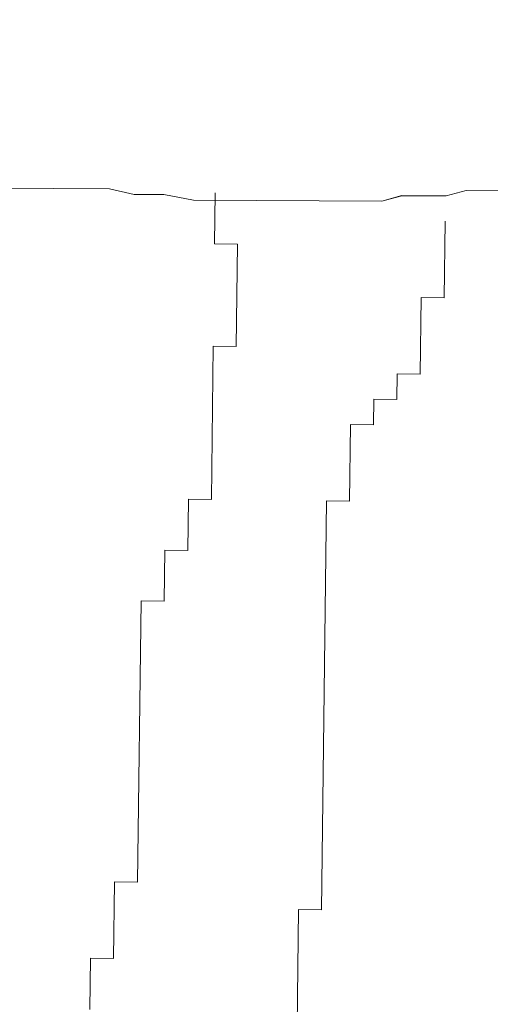
# Model space of a CAD drawing. Units: inches. Extents: x -466983 to 1020, y 324 to 318697.
# Tile 72 of 97: x 647.874 to 650.415, y 942.656 to 947.975. Entities that reach past the tile are written whole.
import ezdxf

# ---------------------------------------------------------------- set-up
doc = ezdxf.new("R2010")
doc.units = ezdxf.units.IN
doc.header["$MEASUREMENT"] = 0
doc.layers.add('A-FLOR-PATT', color=252, linetype='Continuous', lineweight=13)
doc.layers.add('A-FURN', color=8, linetype='Continuous', lineweight=18)

# ---------------------------------------------------------------- blocks, each defined once
blk = doc.blocks.new('L Shaped Sofa')
at = {"ltscale": 2}
for p, q in [((2408.5493, 742.876), (2408.5678, 744.3875)), ((2410.597, 743.3549), (2410.6031, 743.8587)), ((2410.3609, 742.602), (2410.3701, 743.3577)), ((2410.3701, 743.3577), (2410.597, 743.3549)), ((2408.2732, 738.8482), (2408.3225, 742.8788)), ((2408.3225, 742.8788), (2408.5493, 742.876)), ((2410.1002, 739.8337), (2410.1341, 742.6047)), ((2410.1341, 742.6047), (2410.3609, 742.602)), ((2409.8672, 739.3326), (2409.8734, 739.8365)), ((2409.8734, 739.8365), (2410.1002, 739.8337)), ((2409.6342, 738.8316), (2409.6404, 739.3354)), ((2409.6404, 739.3354), (2409.8672, 739.3326)), ((2408.0371, 738.0953), (2408.0464, 738.851)), ((2408.0464, 738.851), (2408.2732, 738.8482)), ((2409.3889, 737.3229), (2409.4074, 738.8344)), ((2409.4074, 738.8344), (2409.6342, 738.8316)), ((2407.8072, 737.8461), (2407.8103, 738.098)), ((2407.8103, 738.098), (2408.0371, 738.0953)), ((2407.5773, 737.597), (2407.5804, 737.8489)), ((2407.5804, 737.8489), (2407.8072, 737.8461)), ((2407.3412, 736.844), (2407.3505, 737.5998)), ((2407.3505, 737.5998), (2407.5773, 737.597)), ((2409.1498, 736.318), (2409.1621, 737.3257)), ((2409.1621, 737.3257), (2409.3889, 737.3229)), ((2407.1052, 736.0911), (2407.1144, 736.8468)), ((2407.1144, 736.8468), (2407.3412, 736.844)), ((2409.3766, 736.3153), (2409.1498, 736.318)), ((2409.3705, 735.8114), (2409.3766, 736.3153)), ((2407.5327, 735.8401), (2407.7282, 735.8934)), ((2407.7282, 735.8934), (2409.5825, 735.8847)), ((2409.5825, 735.8847), (2409.8749, 735.8291)), ((2402.3601, 735.8101), (2406.8981, 735.7888)), ((2406.8981, 735.7888), (2407.0936, 735.8421)), ((2407.0936, 735.8421), (2407.5327, 735.8401)), ((2409.8749, 735.8291), (2410.1677, 735.8277)), ((2410.1677, 735.8277), (2410.4113, 735.7723)), ((2410.4113, 735.7723), (2411.8264, 735.7657))]:
    blk.add_line(p, q, dxfattribs=at)

msp = doc.modelspace()

# ---------------------------------------------------------------- hatches: boundary and pattern name
at = {"layer": 'A-FLOR-PATT', "transparency": 33554572}
h = msp.add_hatch(dxfattribs=at)
h.set_pattern_fill('ANSI37', color=256, scale=30)
h.set_pattern_definition([(45, (-1212.4137, -290.035), (-2.6516504, 2.6516504), []), (135, (-1212.4137, -290.035), (-2.6516504, -2.6516504), [])])
h.paths.add_polyline_path([(901.8057, 1075.9377), (900.6144, 1075.9377), (900.6144, 1065.3856), (899.391, 1065.3856), (898.0911, 1065.3856), (892.8356, 1058.7098, -0.258377), (892.1875, 1058.3509), (879.9848, 1058.3509, -0.20177), (879.4382, 1058.5808), (874.0812, 1065.3856), (872.7813, 1065.3856), (871.5579, 1065.3856), (871.5579, 1075.9377), (813.8057, 1075.9377), (813.8057, 1044.7922), (832.3947, 1044.7922, -0.394795), (848.6602, 1028.5356), (848.6602, 1009.9377), (901.8057, 1009.9377), (901.8057, 1015.9377), (901.3057, 1015.9377), (871.3057, 1015.9377), (871.3057, 1017.2502), (871.3344, 1017.2502, -0.401453), (901.3057, 1045.9377), (901.8057, 1045.9377)])
edge = h.paths.add_edge_path(flags=16)
edge.add_line((847.7731, 1068.9486), (847.7731, 1073.7088))
edge.add_arc((849.2269, 1073.7088), 1.4538, 90, 180, ccw=False)
edge.add_line((849.2269, 1075.1627), (864.4921, 1075.1627))
edge.add_arc((864.4921, 1073.7088), 1.4538, 0, 90, ccw=False)
edge.add_line((865.9459, 1073.7088), (865.9459, 1069.0035))
edge.add_arc((832.6447, 1068.9761), 33.3012, -20.61234, 0.04725, ccw=False)
edge.add_ellipse((856.8595, 1058.48), major_axis=(0, 10.2131), ratio=0.6859192, start_angle=100.00884, end_angle=259.99116, ccw=False)
edge.add_arc((881.0742, 1068.9761), 33.3012, 180.04725, 200.61234, ccw=False)
h.paths.add_polyline_path([(853.1456, 1066.4815), (853.1456, 1066.4534), (853.1463, 1066.4534, 0.433107), (852.9166, 1066.6849), (852.9166, 1066.4534), (853.1456, 1066.4534), (853.1456, 1066.4815), (853.088, 1066.6122, 0.697939), (852.6995, 1066.4534), (852.7003, 1066.4534), (852.7003, 1066.4815), (852.9166, 1067.0012), (852.9166, 1066.6849, -0.396254)], flags=0)
h.paths.add_polyline_path([(861.0187, 1066.4815), (861.0187, 1066.4534), (861.0194, 1066.4534, 0.416404), (860.8024, 1066.6849), (860.8024, 1066.4534), (861.0187, 1066.4534), (861.0187, 1066.4815), (860.9672, 1066.6053, 0.713344), (860.5726, 1066.4534), (860.5734, 1066.4534), (860.5734, 1066.4815), (860.8024, 1067.0012), (860.8024, 1066.6849, -0.379973)], flags=0)
edge = h.paths.add_edge_path(flags=0)
edge.add_spline(control_points=[(861.1298, 1065.7855), (861.4661, 1065.2478), (861.6134, 1065.0161), (861.9833, 1064.3736), (862.1924, 1063.9443), (862.5614, 1063.0391), (862.7212, 1062.5633), (862.9865, 1061.5781), (863.092, 1061.0689), (863.2452, 1060.031), (863.293, 1059.5025), (863.3295, 1058.4409), (863.3181, 1057.9078), (863.2366, 1056.8518), (863.1664, 1056.3289), (862.9695, 1055.308), (862.8427, 1054.8099), (862.5365, 1053.8522), (862.3571, 1053.3927), (861.9514, 1052.5249), (861.7251, 1052.1166), (861.233, 1051.3622), (860.9672, 1051.0162), (860.4048, 1050.3949), (860.1082, 1050.1197), (859.4937, 1049.6461), (859.1758, 1049.4476), (858.5276, 1049.1299), (858.1973, 1049.0107), (857.5315, 1048.8518), (857.1959, 1048.8121), (856.5249, 1048.812), (856.1894, 1048.8515), (855.5236, 1049.0101), (855.1933, 1049.1291), (854.545, 1049.4465), (854.2271, 1049.6449), (853.6124, 1050.1183), (853.3158, 1050.3933), (852.7533, 1051.0143), (852.4874, 1051.3602), (851.9952, 1052.1144), (851.7688, 1052.5225), (851.3629, 1053.3902), (851.1834, 1053.8496), (850.877, 1054.8071), (850.7501, 1055.3051), (850.553, 1056.326), (850.4827, 1056.8488), (850.401, 1057.9048), (850.3895, 1058.4379), (850.4257, 1059.4995), (850.4734, 1060.0281), (850.6265, 1061.066), (850.7318, 1061.5753), (850.9969, 1062.5605), (851.1567, 1063.0365), (851.5254, 1063.9418), (851.7345, 1064.3712), (852.1056, 1065.0164), (852.2544, 1065.2503), (852.6082, 1065.7335)], knot_values=[3.915332, 3.915332, 3.915332, 3.915332, 4.013468, 4.013468, 4.175532, 4.175532, 4.337596, 4.337596, 4.49966, 4.49966, 4.661724, 4.661724, 4.823788, 4.823788, 4.985852, 4.985852, 5.147916, 5.147916, 5.30998, 5.30998, 5.472044, 5.472044, 5.634109, 5.634109, 5.796173, 5.796173, 5.958237, 5.958237, 6.120301, 6.120301, 6.282365, 6.282365, 6.444429, 6.444429, 6.606493, 6.606493, 6.768557, 6.768557, 6.930621, 6.930621, 7.092685, 7.092685, 7.254749, 7.254749, 7.416813, 7.416813, 7.578878, 7.578878, 7.740942, 7.740942, 7.903006, 7.903006, 8.06507, 8.06507, 8.227134, 8.227134, 8.389198, 8.389198, 8.551262, 8.551262, 8.65037, 8.65037, 8.65037, 8.65037], degree=3, periodic=0)
edge.add_line((852.6421, 1065.7855), (861.1298, 1065.7855))
edge = h.paths.add_edge_path(flags=0)
edge.add_ellipse((856.8496, 1057.7432), major_axis=(0, 7.7921), ratio=0.687861, start_angle=0, end_angle=360)
h.paths.add_polyline_path([(848.8634, 1069.3891), (848.8634, 1073.9605, -0.414214), (849.9538, 1075.0508), (863.7652, 1075.0508, -0.414214), (864.8555, 1073.9605), (864.8555, 1069.3891, -0.388936), (864.5237, 1069.027, -0.043561), (849.1953, 1069.027, -0.388936)], flags=0)
h.paths.add_polyline_path([(853.1006, 1068.1122, -1), (852.6775, 1068.1122, -1)], flags=0)
edge = h.paths.add_edge_path(flags=0)
edge.add_ellipse((856.8595, 1057.3378), major_axis=(0, 2.207), ratio=0.657164, start_angle=0, end_angle=360)
h.paths.add_polyline_path([(861.0415, 1068.1122, -1), (860.6184, 1068.1122, -1)], flags=0)
edge = h.paths.add_edge_path()
edge.add_line((573.9537, 1057.3412), (573.9537, 1075.9377))
edge.add_line((573.9537, 1075.9377), (558.7308, 1075.9377))
edge.add_line((558.7308, 1075.9377), (558.7308, 1065.3856))
edge.add_line((558.7308, 1065.3856), (557.5074, 1065.3856))
edge.add_line((557.5074, 1065.3856), (556.2075, 1065.3856))
edge.add_line((556.2075, 1065.3856), (550.952, 1058.7098))
edge.add_arc((550.3039, 1059.1155), 0.7646, 270, 327.9483, ccw=False)
edge.add_line((550.3039, 1058.3509), (538.1012, 1058.3509))
edge.add_arc((538.1012, 1059.1155), 0.7646, 224.3704, 270, ccw=False)
edge.add_line((537.5546, 1058.5808), (532.1976, 1065.3856))
edge.add_line((532.1976, 1065.3856), (530.8977, 1065.3856))
edge.add_line((530.8977, 1065.3856), (529.6743, 1065.3856))
edge.add_line((529.6743, 1065.3856), (529.6743, 1075.9377))
edge.add_line((529.6743, 1075.9377), (520.8057, 1075.9377))
edge.add_line((520.8057, 1075.9377), (520.8057, 1045.9377))
edge.add_line((520.8057, 1045.9377), (521.3057, 1045.9377))
edge.add_arc((521.3057, 1015.9377), 30, 2.50749, 90, ccw=False)
edge.add_line((551.277, 1017.2502), (551.3057, 1017.2502))
edge.add_line((551.3057, 1017.2502), (551.3057, 1015.9377))
edge.add_line((551.3057, 1015.9377), (520.8057, 1015.9377))
edge.add_line((520.8057, 1015.9377), (520.8057, 1009.9377))
edge.add_line((520.8057, 1009.9377), (559.1913, 1010.4022))
edge.add_arc((559.1913, 1011.856), 1.4538, 180, 270, ccw=False)
edge.add_line((557.7375, 1011.856), (557.7375, 1016.5613))
edge.add_arc((591.0386, 1016.5888), 33.3012, 159.38766, 180.04725, ccw=False)
edge.add_ellipse((566.8239, 1027.0848), major_axis=(0, 10.2131), ratio=0.6859192, start_angle=280.00884, end_angle=439.99116, ccw=False)
edge.add_arc((542.6091, 1016.5888), 33.3012, 0.04725, 20.61234, ccw=False)
edge.add_line((575.9103, 1016.6162), (575.9103, 1011.856))
edge.add_arc((574.4565, 1011.856), 1.4538, -90, 0, ccw=False)
edge.add_line((574.4565, 1010.4022), (608.8057, 1009.9377))
edge.add_line((608.8057, 1009.9377), (608.8057, 1041.0857))
edge.add_line((608.8057, 1041.0857), (590.2179, 1041.0857))
edge.add_arc((590.775, 1057.9074), 16.8309, 181.92775, 268.10321, ccw=False)
edge = h.paths.add_edge_path()
edge.add_ellipse((494.2443, 583.6204), major_axis=(0, 10.2131), ratio=0.6859192, start_angle=280.00884, end_angle=439.99116, ccw=False)
edge.add_arc((470.0296, 573.1243), 33.3012, 0.04725, 20.61234, ccw=False)
edge.add_line((503.3307, 573.1518), (503.3307, 568.3916))
edge.add_arc((501.8769, 568.3916), 1.4538, -90, 0, ccw=False)
edge.add_line((501.8769, 566.9377), (539.8057, 566.9377))
edge.add_line((539.8057, 566.9377), (539.8057, 572.9377))
edge.add_line((539.8057, 572.9377), (539.3057, 572.9377))
edge.add_line((539.3057, 572.9377), (509.3057, 572.9377))
edge.add_line((509.3057, 572.9377), (509.3057, 574.2502))
edge.add_line((509.3057, 574.2502), (509.3344, 574.2502))
edge.add_arc((539.3057, 572.9377), 30, 90, 177.49251, ccw=False)
edge.add_line((539.3057, 602.9377), (539.8057, 602.9377))
edge.add_line((539.8057, 602.9377), (539.8057, 626.9377))
edge.add_line((539.8057, 626.9377), (531.7718, 626.9377))
edge.add_line((531.7718, 626.9377), (531.7718, 616.3856))
edge.add_line((531.7718, 616.3856), (530.5484, 616.3856))
edge.add_line((530.5484, 616.3856), (529.2485, 616.3856))
edge.add_line((529.2485, 616.3856), (523.7105, 609.3509))
edge.add_line((523.7105, 609.3509), (510.7766, 609.3509))
edge.add_line((510.7766, 609.3509), (505.2386, 616.3856))
edge.add_line((505.2386, 616.3856), (503.9387, 616.3856))
edge.add_line((503.9387, 616.3856), (502.7153, 616.3856))
edge.add_line((502.7153, 616.3856), (502.7153, 626.9377))
edge.add_line((502.7153, 626.9377), (481.6983, 626.9377))
edge.add_line((481.6983, 626.9377), (481.6983, 610.995))
edge.add_arc((467.2703, 611.4728), 14.4359, 271.92775, 358.10321, ccw=False)
edge.add_line((467.7559, 597.0451), (451.8057, 597.0451))
edge.add_line((451.8057, 597.0451), (451.8057, 584.4035))
edge.add_line((451.8057, 584.4035), (451.8057, 566.9377))
edge.add_line((451.8057, 566.9377), (486.6117, 566.9377))
edge.add_arc((486.6117, 568.3916), 1.4538, 180, 270, ccw=False)
edge.add_line((485.1579, 568.3916), (485.1579, 573.0969))
edge.add_arc((518.4591, 573.1243), 33.3012, 159.38766, 180.04725, ccw=False)
h.paths.add_polyline_path([(836.2609, 1020.7328), (879.8898, 1020.7328), (879.8898, 1039.3902), (836.2609, 1039.3902)], flags=25)
h.paths.add_polyline_path([(549.9851, 1036.7492), (593.614, 1036.7492), (593.614, 1055.4065), (549.9851, 1055.4065)], flags=24)
h.paths.add_polyline_path([(475.123, 595.5959), (518.752, 595.5959), (518.752, 614.2532), (475.123, 614.2532)], flags=24)
h = msp.add_hatch(dxfattribs=at)
h.set_pattern_fill('ANSI37', color=256, scale=20)
h.set_pattern_definition([(45, (-1212.4137, -290.035), (-1.767767, 1.767767), []), (135, (-1212.4137, -290.035), (-1.767767, -1.767767), [])])
h.paths.add_polyline_path([(809.8057, 870.9377), (809.8057, 888.1519), (806.9985, 888.1519), (802.6624, 888.1519), (789.3832, 888.1519), (786.2846, 888.1519, -0.414214), (785.4991, 888.9374), (785.4991, 900.1959), (785.4991, 908.4696, -0.414214), (786.8082, 909.7787, -0.414214), (785.4991, 911.0878), (785.4991, 929.1015, -0.414214), (786.8082, 930.4106, -0.414214), (785.4991, 931.7197), (785.4991, 931.9039, -0.414214), (784.19, 930.5948), (766.7223, 930.5948, -0.412359), (765.4132, 931.8956, -0.413741), (764.1145, 930.5782), (744.5781, 930.422, -0.416556), (743.7864, 931.2075), (743.7864, 933.5153), (742.2154, 933.5153), (742.2154, 952.024, -0.001344), (743.7864, 952.1998), (743.7864, 953.9377), (678.5915, 953.9377), (678.5915, 951.1305), (678.5915, 946.7945), (678.5915, 933.5153), (678.5915, 930.4166, -0.414214), (677.806, 929.6312), (666.5475, 929.6312), (658.2738, 929.6312, -0.414214), (656.9647, 930.9403, -0.414214), (655.6556, 929.6312), (637.6419, 929.6312, -0.414214), (636.3328, 930.9403, -0.414214), (635.0237, 929.6312), (634.8395, 929.6312, -0.414214), (636.1486, 928.322), (636.1486, 910.8544, -0.412359), (634.8478, 909.5452, -0.413741), (636.1653, 908.2466), (636.3214, 888.7102, -0.416556), (635.5359, 887.9184), (633.2281, 887.9184), (633.2281, 886.3475), (614.7194, 886.3475, -0.001344), (614.5436, 887.9184), (612.8057, 887.9184), (612.8057, 834.9377), (612.8057, 752.9377), (612.8057, 748.9377), (612.8057, 697.9377), (654.8057, 697.9377), (654.8057, 701.9377), (715.8057, 701.9377), (715.8057, 737.4353), (774.2918, 737.4353), (774.2918, 795.9377), (809.8057, 795.9377)])
h.paths.add_polyline_path([(679.2761, 849.5757, 0.102523), (682.1475, 849.2608, -0.080461), (694.5428, 849.7725, -0.283899), (694.4822, 849.0082, 0.136605), (694.4068, 848.8103, -0.030441), (694.5428, 846.8929), (694.5428, 842.6198), (694.5428, 838.3466, -0.028219), (694.4246, 836.5684), (694.425, 836.5684, 0.196187), (694.4456, 836.2708, -0.302897), (694.5428, 835.467, -0.080461), (682.1475, 835.9787, 0.102523), (679.2761, 835.6638, -0.58611), (678.6457, 836.0169), (678.6457, 849.2227, -0.58611)], flags=16)
h.paths.add_polyline_path([(679.5173, 848.6515, 0.699597), (679.476, 848.6342, 1.20716), (679.1935, 848.7422, 0.010621)], flags=0)
h.paths.add_polyline_path([(679.4923, 836.5608, -0.013798), (679.9178, 836.6594, -0.071703), (682.8533, 837.1434, -0.165743), (682.1665, 839.1006), (682.1665, 842.6094), (682.1665, 846.0603, -0.240616), (683.4733, 848.6767, -0.068263), (693.9295, 849.0082), (693.7875, 848.7083), (693.7875, 849.0228, 0.067332), (683.4733, 848.6767, 0.240616), (682.1665, 846.0603), (682.1665, 842.6094), (682.1665, 839.1006, 0.23459), (683.461, 836.5513, 0.068093), (693.7875, 836.1955), (693.7875, 836.5104), (693.9296, 836.2102, -0.077215), (682.2421, 836.7815, 0.086627), (679.5283, 836.5701, -0.628402), (679.5029, 836.5735), (679.5029, 836.6071, 0.910458)], flags=0)
h.paths.add_polyline_path([(679.476, 848.6364), (679.2069, 848.647), (679.2069, 836.5718, 0.913566), (679.3645, 836.5861), (679.476, 836.5824)], flags=0)
h.paths.add_polyline_path([(679.2761, 829.8604, 0.102523), (682.1475, 829.5455, -0.080461), (694.5428, 830.0572, -0.283899), (694.4822, 829.2929, 0.136605), (694.4068, 829.095, -0.030441), (694.5428, 827.1776), (694.5428, 822.9045), (694.5428, 818.6314, -0.028219), (694.4246, 816.8531), (694.425, 816.8532, 0.196187), (694.4456, 816.5555, -0.302897), (694.5428, 815.7517, -0.080461), (682.1475, 816.2635, 0.102523), (679.2761, 815.9485, -0.58611), (678.6457, 816.3016), (678.6457, 829.5074, -0.58611)], flags=16)
h.paths.add_polyline_path([(679.5173, 828.9362, 0.699597), (679.476, 828.9189, 1.20716), (679.1935, 829.0269, 0.010621)], flags=0)
h.paths.add_polyline_path([(679.4923, 816.8456, -0.013798), (679.9178, 816.9441, -0.071703), (682.8533, 817.4281, -0.165743), (682.1665, 819.3853), (682.1665, 822.8941), (682.1665, 826.345, -0.240616), (683.4733, 828.9614, -0.068263), (693.9295, 829.2929), (693.7875, 828.9931), (693.7875, 829.3076, 0.067332), (683.4733, 828.9614, 0.240616), (682.1665, 826.345), (682.1665, 822.8941), (682.1665, 819.3853, 0.23459), (683.461, 816.836, 0.068093), (693.7875, 816.4802), (693.7875, 816.7952), (693.9296, 816.4949, -0.077215), (682.2421, 817.0662, 0.086627), (679.5283, 816.8549, -0.628402), (679.5029, 816.8582), (679.5029, 816.8918, 0.910458)], flags=0)
h.paths.add_polyline_path([(679.476, 828.9211), (679.2069, 828.9317), (679.2069, 816.8565, 0.913566), (679.3645, 816.8708), (679.476, 816.8671)], flags=0)
h.paths.add_polyline_path([(679.2761, 810.1451, 0.102523), (682.1475, 809.8302, -0.080461), (694.5428, 810.342, -0.3023), (694.4466, 809.5394, 0.10023), (694.4058, 809.3878, -0.03057), (694.5428, 807.4623), (694.5428, 803.1892), (694.5428, 798.9161, -0.03057), (694.4058, 796.9906, 0.10023), (694.4466, 796.839, -0.3023), (694.5428, 796.0365, -0.080461), (682.1475, 796.5482, 0.102523), (679.2761, 796.2333, -0.58611), (678.6457, 796.5863), (678.6457, 809.7921, -0.58611)], flags=16)
h.paths.add_polyline_path([(679.5173, 809.2417, 0.699597), (679.476, 809.2244, 1.20716), (679.1935, 809.3324, 0.010621)], flags=0)
h.paths.add_polyline_path([(679.4923, 797.151, -0.013798), (679.9178, 797.2496, -0.071703), (682.8533, 797.7336, -0.165743), (682.1665, 799.6908), (682.1665, 803.1996), (682.1665, 806.6505, -0.239349), (683.461, 809.2577, -0.072465), (694.4468, 809.5405, 0.197932), (694.425, 809.2405), (693.7875, 809.2985), (693.7875, 809.6135, 0.068093), (683.461, 809.2577, 0.239349), (682.1665, 806.6505), (682.1665, 803.1996), (682.1665, 799.6908, 0.235854), (683.4733, 797.1323, 0.067332), (693.7875, 796.7861), (693.7875, 797.1006), (694.425, 797.1586, 0.197932), (694.4468, 796.8586, -0.080419), (682.1557, 797.3795, 0.083867), (679.5283, 797.1603, -0.628402), (679.5029, 797.1637), (679.5029, 797.1973, 0.910458)], flags=0)
h.paths.add_polyline_path([(679.2069, 809.2372), (679.2069, 797.162, 0.913566), (679.3645, 797.1763), (679.476, 797.1726), (679.476, 809.2266)], flags=0)
h.paths.add_polyline_path([(695.3643, 853.2989), (728.2231, 853.2989), (728.2231, 771.1519), (695.3643, 771.1519)], flags=16)
h.paths.add_polyline_path([(696.0215, 852.6417), (727.5659, 852.6417), (727.5659, 771.809), (696.0215, 771.809)], flags=0)
h.paths.add_polyline_path([(679.2761, 788.7869, 0.102523), (682.1475, 788.472, -0.080461), (694.5428, 788.9837, -0.3023), (694.4466, 788.1812, 0.10023), (694.4058, 788.0296, -0.03057), (694.5428, 786.1041), (694.5428, 781.831), (694.5428, 777.5578, -0.03057), (694.4058, 775.6323, 0.10023), (694.4466, 775.4808, -0.3023), (694.5428, 774.6782, -0.080461), (682.1475, 775.19, 0.102523), (679.2761, 774.875, -0.58611), (678.6457, 775.2281), (678.6457, 788.4339, -0.58611)], flags=16)
h.paths.add_polyline_path([(679.5173, 787.8834, 0.699597), (679.476, 787.8662, 1.20716), (679.1935, 787.9742, 0.010621)], flags=0)
h.paths.add_polyline_path([(679.4923, 775.7928, -0.013798), (679.9178, 775.8914, -0.071703), (682.8533, 776.3753, -0.165743), (682.1665, 778.3325), (682.1665, 781.8414), (682.1665, 785.2922, -0.239349), (683.461, 787.8995, -0.072465), (694.4468, 788.1823, 0.197932), (694.425, 787.8823), (693.7875, 787.9403), (693.7875, 788.2553, 0.068093), (683.461, 787.8995, 0.239349), (682.1665, 785.2922), (682.1665, 781.8414), (682.1665, 778.3325, 0.235854), (683.4733, 775.7741, 0.067332), (693.7875, 775.4279), (693.7875, 775.7424), (694.425, 775.8004, 0.197932), (694.4468, 775.5004, -0.080419), (682.1557, 776.0212, 0.083867), (679.5283, 775.8021, -0.628402), (679.5029, 775.8054), (679.5029, 775.8391, 0.910458)], flags=0)
h.paths.add_polyline_path([(679.2069, 787.8789), (679.2069, 775.8038, 0.913566), (679.3645, 775.818), (679.476, 775.8144), (679.476, 787.8684)], flags=0)
h.paths.add_polyline_path([(704.641, 854.1204, -0.080461), (705.1527, 866.5157, 0.102523), (704.8378, 869.3871, -0.58611), (705.1908, 870.0174), (718.3966, 870.0174, -0.58611), (718.7496, 869.3871, 0.102523), (718.4347, 866.5157, -0.080461), (718.9465, 854.1204, -0.3023), (718.1439, 854.2166, 0.10023), (717.9924, 854.2574, -0.03057), (716.0668, 854.1204), (711.7937, 854.1204), (707.5206, 854.1204, -0.03057), (705.5951, 854.2574, 0.10023), (705.4435, 854.2166, -0.3023)], flags=16)
h.paths.add_polyline_path([(717.8462, 869.1459, 0.699597), (717.8289, 869.1872, 1.20716), (717.9369, 869.4697, 0.010621)], flags=0)
h.paths.add_polyline_path([(705.4631, 854.2164, -0.080419), (705.984, 866.5074, 0.083867), (705.7648, 869.1349, -0.628402), (705.7682, 869.1603), (705.8018, 869.1603, 0.910458), (705.7555, 869.1709, -0.013798), (705.8541, 868.7454, -0.071703), (706.3381, 865.8099, -0.165743), (708.2953, 866.4967), (711.8041, 866.4967), (715.255, 866.4967, -0.239349), (717.8622, 865.2022, -0.072465), (718.145, 854.2164, 0.197932), (717.845, 854.2382), (717.903, 854.8757), (718.218, 854.8757, 0.068093), (717.8622, 865.2022, 0.239349), (715.255, 866.4967), (711.8041, 866.4967), (708.2953, 866.4967, 0.235854), (705.7368, 865.1898, 0.067332), (705.3906, 854.8757), (705.7051, 854.8757), (705.7631, 854.2382, 0.197932)], flags=16)
h.paths.add_polyline_path([(705.7665, 869.4563, 0.913566), (705.7808, 869.2987), (705.7771, 869.1872), (717.8311, 869.1872), (717.8417, 869.4563)], flags=0)
h.paths.add_polyline_path([(729.0446, 842.6198), (729.0446, 846.8929, -0.03057), (729.1817, 848.8184, 0.10023), (729.1408, 848.9699, -0.3023), (729.0446, 849.7725, -0.080461), (741.4399, 849.2608, 0.102523), (744.3113, 849.5757, -0.58611), (744.9417, 849.2227), (744.9417, 836.0169, -0.58611), (744.3113, 835.6638, 0.102523), (741.4399, 835.9787, -0.080461), (729.0446, 835.467, -0.3023), (729.1408, 836.2696, 0.10023), (729.1817, 836.4211, -0.03057), (729.0446, 838.3466)], flags=16)
h.paths.add_polyline_path([(744.1115, 836.5846, 1.20716), (744.3939, 836.4766, 0.010621), (744.0701, 836.5673, 0.699597)], flags=0)
h.paths.add_polyline_path([(729.1407, 836.2684, 0.197932), (729.1624, 836.5684), (729.7999, 836.5104), (729.7999, 836.1955, 0.068093), (740.1264, 836.5513, 0.239349), (741.4209, 839.1585), (741.4209, 842.6094), (741.4209, 846.1182, 0.235854), (740.1141, 848.6767, 0.067332), (729.7999, 849.0228), (729.7999, 848.7083), (729.1624, 848.6503, 0.197932), (729.1407, 848.9504, -0.080419), (741.4317, 848.4295, 0.083867), (744.0591, 848.6486, -0.628402), (744.0845, 848.6453), (744.0845, 848.6117, 0.910458), (744.0951, 848.6579, -0.013798), (743.6696, 848.5594, -0.071703), (740.7341, 848.0754, -0.165743), (741.4209, 846.1182), (741.4209, 842.6094), (741.4209, 839.1585, -0.239349), (740.1264, 836.5513, -0.072465)], flags=0)
h.paths.add_polyline_path([(729.0446, 830.0572, -0.080461), (741.4399, 829.5455, 0.102523), (744.3113, 829.8604, -0.58611), (744.9417, 829.5074), (744.9417, 816.3016, -0.58611), (744.3113, 815.9485, 0.102523), (741.4399, 816.2635, -0.080461), (729.0446, 815.7517, -0.3023), (729.1408, 816.5543, 0.10023), (729.1817, 816.7058, -0.03057), (729.0446, 818.6314), (729.0446, 822.9045), (729.0446, 827.1776, -0.03057), (729.1817, 829.1031, 0.10023), (729.1408, 829.2547, -0.3023)], flags=16)
h.paths.add_polyline_path([(744.1115, 816.8693, 1.20716), (744.3939, 816.7613, 0.010621), (744.0701, 816.852, 0.699597)], flags=0)
h.paths.add_polyline_path([(729.1407, 829.2351, -0.080419), (741.4317, 828.7142, 0.083867), (744.0591, 828.9334, -0.628402), (744.0845, 828.93), (744.0845, 828.8964, 0.910458), (744.0951, 828.9427, -0.013798), (743.6696, 828.8441, -0.071703), (740.7341, 828.3601, -0.165743), (741.4209, 826.4029), (741.4209, 822.8941), (741.4209, 819.4432, -0.239349), (740.1264, 816.836, -0.072465), (729.1407, 816.5531, 0.197932), (729.1624, 816.8532), (729.7999, 816.7952), (729.7999, 816.4802, 0.068093), (740.1264, 816.836, 0.239349), (741.4209, 819.4432), (741.4209, 822.8941), (741.4209, 826.4029, 0.235854), (740.1141, 828.9614, 0.067332), (729.7999, 829.3076), (729.7999, 828.9931), (729.1624, 828.9351, 0.197932)], flags=16)
h.paths.add_polyline_path([(729.0446, 810.342, -0.080461), (741.4399, 809.8302, 0.102523), (744.3113, 810.1451, -0.58611), (744.9417, 809.7921), (744.9417, 796.5863, -0.58611), (744.3113, 796.2333, 0.102523), (741.4399, 796.5482, -0.080461), (729.0446, 796.0365, -0.283899), (729.1052, 796.8007, 0.136605), (729.1806, 796.9987, -0.030441), (729.0446, 798.9161), (729.0446, 803.1892), (729.0446, 807.4623, -0.028219), (729.1628, 809.2406), (729.1624, 809.2405, 0.196187), (729.1418, 809.5382, -0.302897)], flags=16)
h.paths.add_polyline_path([(744.1115, 797.1748, 1.20716), (744.3939, 797.0668, 0.010621), (744.0701, 797.1575, 0.699597)], flags=0)
h.paths.add_polyline_path([(741.3453, 809.0275, 0.086627), (744.0591, 809.2388, -0.628402), (744.0845, 809.2355), (744.0845, 809.2019, 0.910458), (744.0951, 809.2481, -0.013798), (743.6696, 809.1496, -0.071703), (740.7341, 808.6656, -0.165743), (741.4209, 806.7084), (741.4209, 803.1996), (741.4209, 799.7487, -0.240616), (740.1141, 797.1323, -0.068263), (729.658, 796.8008), (729.7999, 797.1006), (729.7999, 796.7861, 0.067332), (740.1141, 797.1323, 0.240616), (741.4209, 799.7487), (741.4209, 803.1996), (741.4209, 806.7084, 0.23459), (740.1264, 809.2577, 0.068093), (729.7999, 809.6135), (729.7999, 809.2985), (729.6578, 809.5988, -0.077215)], flags=0)
h.paths.add_polyline_path([(704.641, 770.3304, -0.283899), (705.4053, 770.2697, 0.136605), (705.6032, 770.1944, -0.030441), (707.5206, 770.3304), (711.7937, 770.3304), (716.0668, 770.3304, -0.028219), (717.8451, 770.2122), (717.845, 770.2126, 0.196187), (718.1427, 770.2331, -0.302897), (718.9465, 770.3304, -0.080461), (718.4347, 757.9351, 0.102523), (718.7496, 755.0637, -0.58611), (718.3966, 754.4333), (705.1908, 754.4333, -0.58611), (704.8378, 755.0637, 0.102523), (705.1527, 757.9351, -0.080461)], flags=16)
h.paths.add_polyline_path([(705.762, 755.3048, 0.699597), (705.7793, 755.2635, 1.20716), (705.6713, 754.9811, 0.010621)], flags=0)
h.paths.add_polyline_path([(705.4053, 769.717), (705.7051, 769.5751), (705.3906, 769.5751, 0.067332), (705.7368, 759.2609, 0.240616), (708.3532, 757.954), (711.8041, 757.954), (715.3129, 757.954, 0.23459), (717.8622, 759.2485, 0.068093), (718.218, 769.5751), (717.903, 769.5751), (718.2033, 769.7172, -0.077215), (717.632, 758.0297, 0.086627), (717.8433, 755.3159, -0.628402), (717.84, 755.2904), (717.8064, 755.2904, 0.910458), (717.8526, 755.2799, -0.013798), (717.7541, 755.7053, -0.071703), (717.2701, 758.6409, -0.165743), (715.3129, 757.954), (711.8041, 757.954), (708.3532, 757.954, -0.240616), (705.7368, 759.2609, -0.068263)], flags=0)
h.paths.add_polyline_path([(729.0446, 788.9837, -0.080461), (741.4399, 788.472, 0.102523), (744.3113, 788.7869, -0.58611), (744.9417, 788.4339), (744.9417, 775.2281, -0.58611), (744.3113, 774.875, 0.102523), (741.4399, 775.19, -0.080461), (729.0446, 774.6782, -0.283899), (729.1052, 775.4425, 0.136605), (729.1806, 775.6405, -0.030441), (729.0446, 777.5578), (729.0446, 781.831), (729.0446, 786.1041, -0.028219), (729.1628, 787.8823), (729.1624, 787.8823, 0.196187), (729.1418, 788.1799, -0.302897)], flags=16)
h.paths.add_polyline_path([(744.1115, 775.8165, 1.20716), (744.3939, 775.7086, 0.010621), (744.0701, 775.7993, 0.699597)], flags=0)
h.paths.add_polyline_path([(741.3453, 787.6692, 0.086627), (744.0591, 787.8806, -0.628402), (744.0845, 787.8773), (744.0845, 787.8437, 0.910458), (744.0951, 787.8899, -0.013798), (743.6696, 787.7913, -0.071703), (740.7341, 787.3074, -0.165743), (741.4209, 785.3502), (741.4209, 781.8414), (741.4209, 778.3905, -0.240616), (740.1141, 775.7741, -0.068263), (729.658, 775.4425), (729.7999, 775.7424), (729.7999, 775.4279, 0.067332), (740.1141, 775.7741, 0.240616), (741.4209, 778.3905), (741.4209, 781.8414), (741.4209, 785.3502, 0.23459), (740.1264, 787.8995, 0.068093), (729.7999, 788.2553), (729.7999, 787.9403), (729.6578, 788.2405, -0.077215)], flags=0)
h.paths.add_polyline_path([(744.1115, 848.6364), (744.1115, 836.5824), (744.3805, 836.5718), (744.3805, 848.647, 0.913566), (744.2229, 848.6327)], flags=0)
h.paths.add_polyline_path([(744.2229, 828.9174), (744.1115, 828.9211), (744.1115, 816.8671), (744.3805, 816.8565), (744.3805, 828.9317, 0.913566)], flags=0)
h.paths.add_polyline_path([(717.8311, 755.2635), (705.7771, 755.2635), (705.7665, 754.9945), (717.8417, 754.9945, 0.913566), (717.8274, 755.1521)], flags=0)
h.paths.add_polyline_path([(744.2229, 809.2229), (744.1115, 809.2266), (744.1115, 797.1726), (744.3805, 797.162), (744.3805, 809.2372, 0.913566)], flags=0)
h.paths.add_polyline_path([(744.1115, 787.8684), (744.1115, 775.8144), (744.3805, 775.8038), (744.3805, 787.8789, 0.913566), (744.2229, 787.8647)], flags=0)
h.paths.add_polyline_path([(678.8774, 877.1228), (737.6127, 877.1228), (737.6127, 899.5116), (678.8774, 899.5116)], flags=24)

# ---------------------------------------------------------------- linework, layer by layer
at = {"layer": 'A-FURN', "ltscale": 2}
for p, q in [((648.3583, 947.0615), (647.5825, 947.0651)), ((648.3583, 947.0615), (647.5825, 947.0651)), ((648.3583, 947.0615), (647.5825, 947.0651)), ((648.3583, 947.0615), (647.5825, 947.0651)), ((648.3583, 947.0615), (647.5825, 947.0651)), ((648.3583, 947.0615), (647.5825, 947.0651)), ((648.4918, 947.0312), (648.3583, 947.0615)), ((648.4918, 947.0312), (648.3583, 947.0615)), ((648.4918, 947.0312), (648.3583, 947.0615)), ((648.4918, 947.0312), (648.3583, 947.0615)), ((648.4918, 947.0312), (648.3583, 947.0615)), ((648.4918, 947.0312), (648.3583, 947.0615)), ((650.2843, 947.0525), (650.1771, 947.0232)), ((650.2843, 947.0525), (650.1771, 947.0232)), ((650.2843, 947.0525), (650.1771, 947.0232)), ((650.2843, 947.0525), (650.1771, 947.0232)), ((650.2843, 947.0525), (650.1771, 947.0232)), ((650.2843, 947.0525), (650.1771, 947.0232)), ((652.7721, 947.0408), (650.2843, 947.0525)), ((652.7721, 947.0408), (650.2843, 947.0525)), ((652.7721, 947.0408), (650.2843, 947.0525)), ((652.7721, 947.0408), (650.2843, 947.0525)), ((652.7721, 947.0408), (650.2843, 947.0525)), ((652.7721, 947.0408), (650.2843, 947.0525)), ((648.6523, 947.0304), (648.4918, 947.0312)), ((648.6523, 947.0304), (648.4918, 947.0312)), ((648.6523, 947.0304), (648.4918, 947.0312)), ((648.6523, 947.0304), (648.4918, 947.0312)), ((648.6523, 947.0304), (648.4918, 947.0312)), ((648.6523, 947.0304), (648.4918, 947.0312)), ((648.8127, 946.9999), (648.6523, 947.0304)), ((648.8127, 946.9999), (648.6523, 947.0304)), ((648.8127, 946.9999), (648.6523, 947.0304)), ((648.8127, 946.9999), (648.6523, 947.0304)), ((648.8127, 946.9999), (648.6523, 947.0304)), ((648.8127, 946.9999), (648.6523, 947.0304)), ((649.8292, 946.9952), (648.8127, 946.9999)), ((649.8292, 946.9952), (648.8127, 946.9999)), ((649.8292, 946.9952), (648.8127, 946.9999)), ((649.8292, 946.9952), (648.8127, 946.9999)), ((649.8292, 946.9952), (648.8127, 946.9999)), ((649.8292, 946.9952), (648.8127, 946.9999)), ((648.9289, 947.0401), (648.9255, 946.7639)), ((648.9289, 947.0401), (648.9255, 946.7639)), ((648.9289, 947.0401), (648.9255, 946.7639)), ((648.9289, 947.0401), (648.9255, 946.7639)), ((648.9289, 947.0401), (648.9255, 946.7639)), ((648.9289, 947.0401), (648.9255, 946.7639)), ((649.9363, 947.0244), (649.8292, 946.9952)), ((649.9363, 947.0244), (649.8292, 946.9952)), ((649.9363, 947.0244), (649.8292, 946.9952)), ((649.9363, 947.0244), (649.8292, 946.9952)), ((649.9363, 947.0244), (649.8292, 946.9952)), ((649.9363, 947.0244), (649.8292, 946.9952)), ((650.1771, 947.0232), (649.9363, 947.0244)), ((650.1771, 947.0232), (649.9363, 947.0244)), ((650.1771, 947.0232), (649.9363, 947.0244)), ((650.1771, 947.0232), (649.9363, 947.0244)), ((650.1771, 947.0232), (649.9363, 947.0244)), ((650.1771, 947.0232), (649.9363, 947.0244)), ((650.1707, 946.8868), (650.1657, 946.4725)), ((650.1707, 946.8868), (650.1657, 946.4725)), ((650.1707, 946.8868), (650.1657, 946.4725)), ((650.1707, 946.8868), (650.1657, 946.4725)), ((650.1707, 946.8868), (650.1657, 946.4725)), ((650.1707, 946.8868), (650.1657, 946.4725)), ((648.9255, 946.7639), (649.0499, 946.7624)), ((648.9255, 946.7639), (649.0499, 946.7624)), ((648.9255, 946.7639), (649.0499, 946.7624)), ((648.9255, 946.7639), (649.0499, 946.7624)), ((648.9255, 946.7639), (649.0499, 946.7624)), ((648.9255, 946.7639), (649.0499, 946.7624)), ((649.0499, 946.7624), (649.0431, 946.2099)), ((649.0499, 946.7624), (649.0431, 946.2099)), ((649.0499, 946.7624), (649.0431, 946.2099)), ((649.0499, 946.7624), (649.0431, 946.2099)), ((649.0499, 946.7624), (649.0431, 946.2099)), ((649.0499, 946.7624), (649.0431, 946.2099)), ((650.0413, 946.474), (650.0363, 946.0597)), ((650.0413, 946.474), (650.0363, 946.0597)), ((650.0413, 946.474), (650.0363, 946.0597)), ((650.0413, 946.474), (650.0363, 946.0597)), ((650.0413, 946.474), (650.0363, 946.0597)), ((650.0413, 946.474), (650.0363, 946.0597)), ((650.1657, 946.4725), (650.0413, 946.474)), ((650.1657, 946.4725), (650.0413, 946.474)), ((650.1657, 946.4725), (650.0413, 946.474)), ((650.1657, 946.4725), (650.0413, 946.474)), ((650.1657, 946.4725), (650.0413, 946.474)), ((650.1657, 946.4725), (650.0413, 946.474)), ((648.9188, 946.2115), (648.9086, 945.3829)), ((648.9188, 946.2115), (648.9086, 945.3829)), ((648.9188, 946.2115), (648.9086, 945.3829)), ((648.9188, 946.2115), (648.9086, 945.3829)), ((648.9188, 946.2115), (648.9086, 945.3829)), ((648.9188, 946.2115), (648.9086, 945.3829)), ((649.0431, 946.2099), (648.9188, 946.2115)), ((649.0431, 946.2099), (648.9188, 946.2115)), ((649.0431, 946.2099), (648.9188, 946.2115)), ((649.0431, 946.2099), (648.9188, 946.2115)), ((649.0431, 946.2099), (648.9188, 946.2115)), ((649.0431, 946.2099), (648.9188, 946.2115)), ((649.9119, 946.0612), (649.9102, 945.9231)), ((649.9119, 946.0612), (649.9102, 945.9231)), ((649.9119, 946.0612), (649.9102, 945.9231)), ((649.9119, 946.0612), (649.9102, 945.9231)), ((649.9119, 946.0612), (649.9102, 945.9231)), ((649.9119, 946.0612), (649.9102, 945.9231)), ((650.0363, 946.0597), (649.9119, 946.0612)), ((650.0363, 946.0597), (649.9119, 946.0612)), ((650.0363, 946.0597), (649.9119, 946.0612)), ((650.0363, 946.0597), (649.9119, 946.0612)), ((650.0363, 946.0597), (649.9119, 946.0612)), ((650.0363, 946.0597), (649.9119, 946.0612)), ((649.7859, 945.9246), (649.7842, 945.7865)), ((649.7859, 945.9246), (649.7842, 945.7865)), ((649.7859, 945.9246), (649.7842, 945.7865)), ((649.7859, 945.9246), (649.7842, 945.7865)), ((649.7859, 945.9246), (649.7842, 945.7865)), ((649.7859, 945.9246), (649.7842, 945.7865)), ((649.9102, 945.9231), (649.7859, 945.9246)), ((649.9102, 945.9231), (649.7859, 945.9246)), ((649.9102, 945.9231), (649.7859, 945.9246)), ((649.9102, 945.9231), (649.7859, 945.9246)), ((649.9102, 945.9231), (649.7859, 945.9246)), ((649.9102, 945.9231), (649.7859, 945.9246)), ((649.6598, 945.788), (649.6548, 945.3737)), ((649.6598, 945.788), (649.6548, 945.3737)), ((649.6598, 945.788), (649.6548, 945.3737)), ((649.6598, 945.788), (649.6548, 945.3737)), ((649.6598, 945.788), (649.6548, 945.3737)), ((649.6598, 945.788), (649.6548, 945.3737)), ((649.7842, 945.7865), (649.6598, 945.788)), ((649.7842, 945.7865), (649.6598, 945.788)), ((649.7842, 945.7865), (649.6598, 945.788)), ((649.7842, 945.7865), (649.6598, 945.788)), ((649.7842, 945.7865), (649.6598, 945.788)), ((649.7842, 945.7865), (649.6598, 945.788)), ((648.7843, 945.3844), (648.7809, 945.1082)), ((648.7843, 945.3844), (648.7809, 945.1082)), ((648.7843, 945.3844), (648.7809, 945.1082)), ((648.7843, 945.3844), (648.7809, 945.1082)), ((648.7843, 945.3844), (648.7809, 945.1082)), ((648.7843, 945.3844), (648.7809, 945.1082)), ((648.9086, 945.3829), (648.7843, 945.3844)), ((648.9086, 945.3829), (648.7843, 945.3844)), ((648.9086, 945.3829), (648.7843, 945.3844)), ((648.9086, 945.3829), (648.7843, 945.3844)), ((648.9086, 945.3829), (648.7843, 945.3844)), ((648.9086, 945.3829), (648.7843, 945.3844)), ((649.5304, 945.3753), (649.5034, 943.1656)), ((649.5304, 945.3753), (649.5034, 943.1656)), ((649.5304, 945.3753), (649.5034, 943.1656)), ((649.5304, 945.3753), (649.5034, 943.1656)), ((649.5304, 945.3753), (649.5034, 943.1656)), ((649.5304, 945.3753), (649.5034, 943.1656)), ((649.6548, 945.3737), (649.5304, 945.3753)), ((649.6548, 945.3737), (649.5304, 945.3753)), ((649.6548, 945.3737), (649.5304, 945.3753)), ((649.6548, 945.3737), (649.5304, 945.3753)), ((649.6548, 945.3737), (649.5304, 945.3753)), ((649.6548, 945.3737), (649.5304, 945.3753)), ((648.6565, 945.1097), (648.6532, 944.8335)), ((648.6565, 945.1097), (648.6532, 944.8335)), ((648.6565, 945.1097), (648.6532, 944.8335)), ((648.6565, 945.1097), (648.6532, 944.8335)), ((648.6565, 945.1097), (648.6532, 944.8335)), ((648.6565, 945.1097), (648.6532, 944.8335)), ((648.7809, 945.1082), (648.6565, 945.1097)), ((648.7809, 945.1082), (648.6565, 945.1097)), ((648.7809, 945.1082), (648.6565, 945.1097)), ((648.7809, 945.1082), (648.6565, 945.1097)), ((648.7809, 945.1082), (648.6565, 945.1097)), ((648.7809, 945.1082), (648.6565, 945.1097)), ((648.5288, 944.835), (648.5103, 943.3159)), ((648.5288, 944.835), (648.5103, 943.3159)), ((648.5288, 944.835), (648.5103, 943.3159)), ((648.5288, 944.835), (648.5103, 943.3159)), ((648.5288, 944.835), (648.5103, 943.3159)), ((648.5288, 944.835), (648.5103, 943.3159)), ((648.6532, 944.8335), (648.5288, 944.835)), ((648.6532, 944.8335), (648.5288, 944.835)), ((648.6532, 944.8335), (648.5288, 944.835)), ((648.6532, 944.8335), (648.5288, 944.835)), ((648.6532, 944.8335), (648.5288, 944.835)), ((648.6532, 944.8335), (648.5288, 944.835)), ((648.3859, 943.3174), (648.3808, 942.9031)), ((648.3859, 943.3174), (648.3808, 942.9031)), ((648.3859, 943.3174), (648.3808, 942.9031)), ((648.3859, 943.3174), (648.3808, 942.9031)), ((648.3859, 943.3174), (648.3808, 942.9031)), ((648.3859, 943.3174), (648.3808, 942.9031)), ((648.5103, 943.3159), (648.3859, 943.3174)), ((648.5103, 943.3159), (648.3859, 943.3174)), ((648.5103, 943.3159), (648.3859, 943.3174)), ((648.5103, 943.3159), (648.3859, 943.3174)), ((648.5103, 943.3159), (648.3859, 943.3174)), ((648.5103, 943.3159), (648.3859, 943.3174)), ((649.3791, 943.1671), (649.3689, 942.3385)), ((649.3791, 943.1671), (649.3689, 942.3385)), ((649.3791, 943.1671), (649.3689, 942.3385)), ((649.3791, 943.1671), (649.3689, 942.3385)), ((649.3791, 943.1671), (649.3689, 942.3385)), ((649.3791, 943.1671), (649.3689, 942.3385)), ((649.5034, 943.1656), (649.3791, 943.1671)), ((649.5034, 943.1656), (649.3791, 943.1671)), ((649.5034, 943.1656), (649.3791, 943.1671)), ((649.5034, 943.1656), (649.3791, 943.1671)), ((649.5034, 943.1656), (649.3791, 943.1671)), ((649.5034, 943.1656), (649.3791, 943.1671)), ((648.2565, 942.9046), (648.2531, 942.6284)), ((648.2565, 942.9046), (648.2531, 942.6284)), ((648.2565, 942.9046), (648.2531, 942.6284)), ((648.2565, 942.9046), (648.2531, 942.6284)), ((648.2565, 942.9046), (648.2531, 942.6284)), ((648.2565, 942.9046), (648.2531, 942.6284)), ((648.3808, 942.9031), (648.2565, 942.9046)), ((648.3808, 942.9031), (648.2565, 942.9046)), ((648.3808, 942.9031), (648.2565, 942.9046)), ((648.3808, 942.9031), (648.2565, 942.9046)), ((648.3808, 942.9031), (648.2565, 942.9046)), ((648.3808, 942.9031), (648.2565, 942.9046))]:
    msp.add_line(p, q, dxfattribs=at)

# ---------------------------------------------------------------- block references
at = {"layer": 'A-FURN', "xscale": 0.5482153745360612, "yscale": 0.5482153745360612, "zscale": 0.5482153745360612, "rotation": 180}
msp.add_blockref('L Shaped Sofa', (1969.7828, 1350.4232), dxfattribs=at)

doc.saveas('drawing.dxf')
